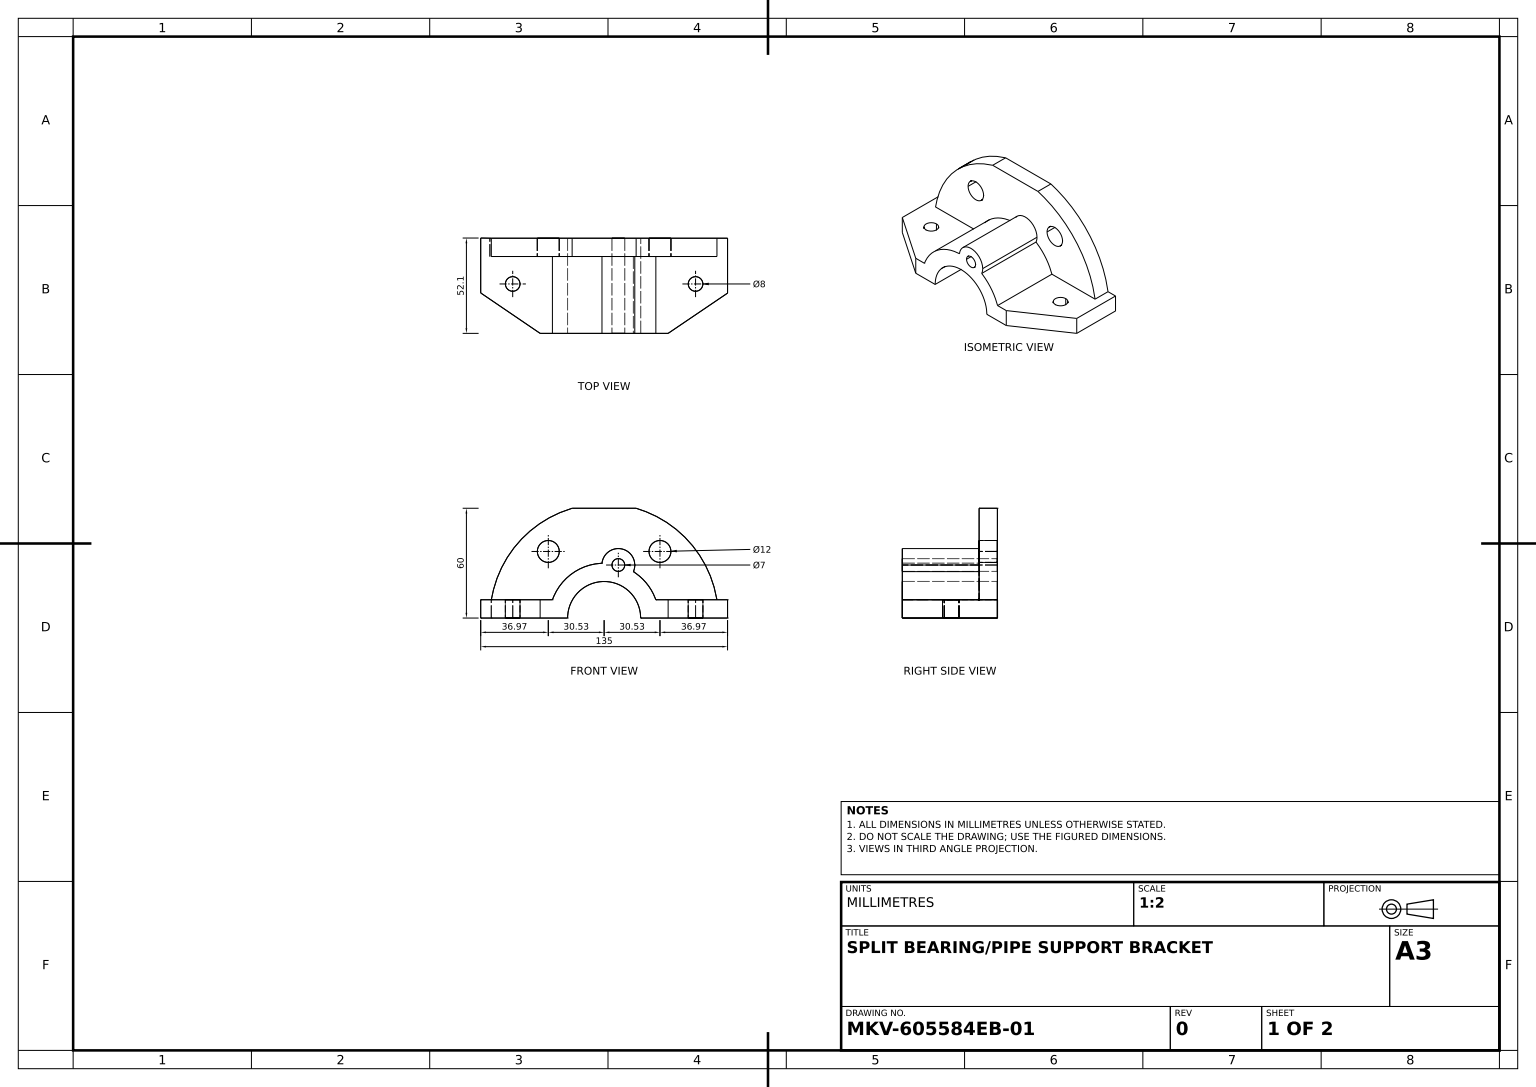
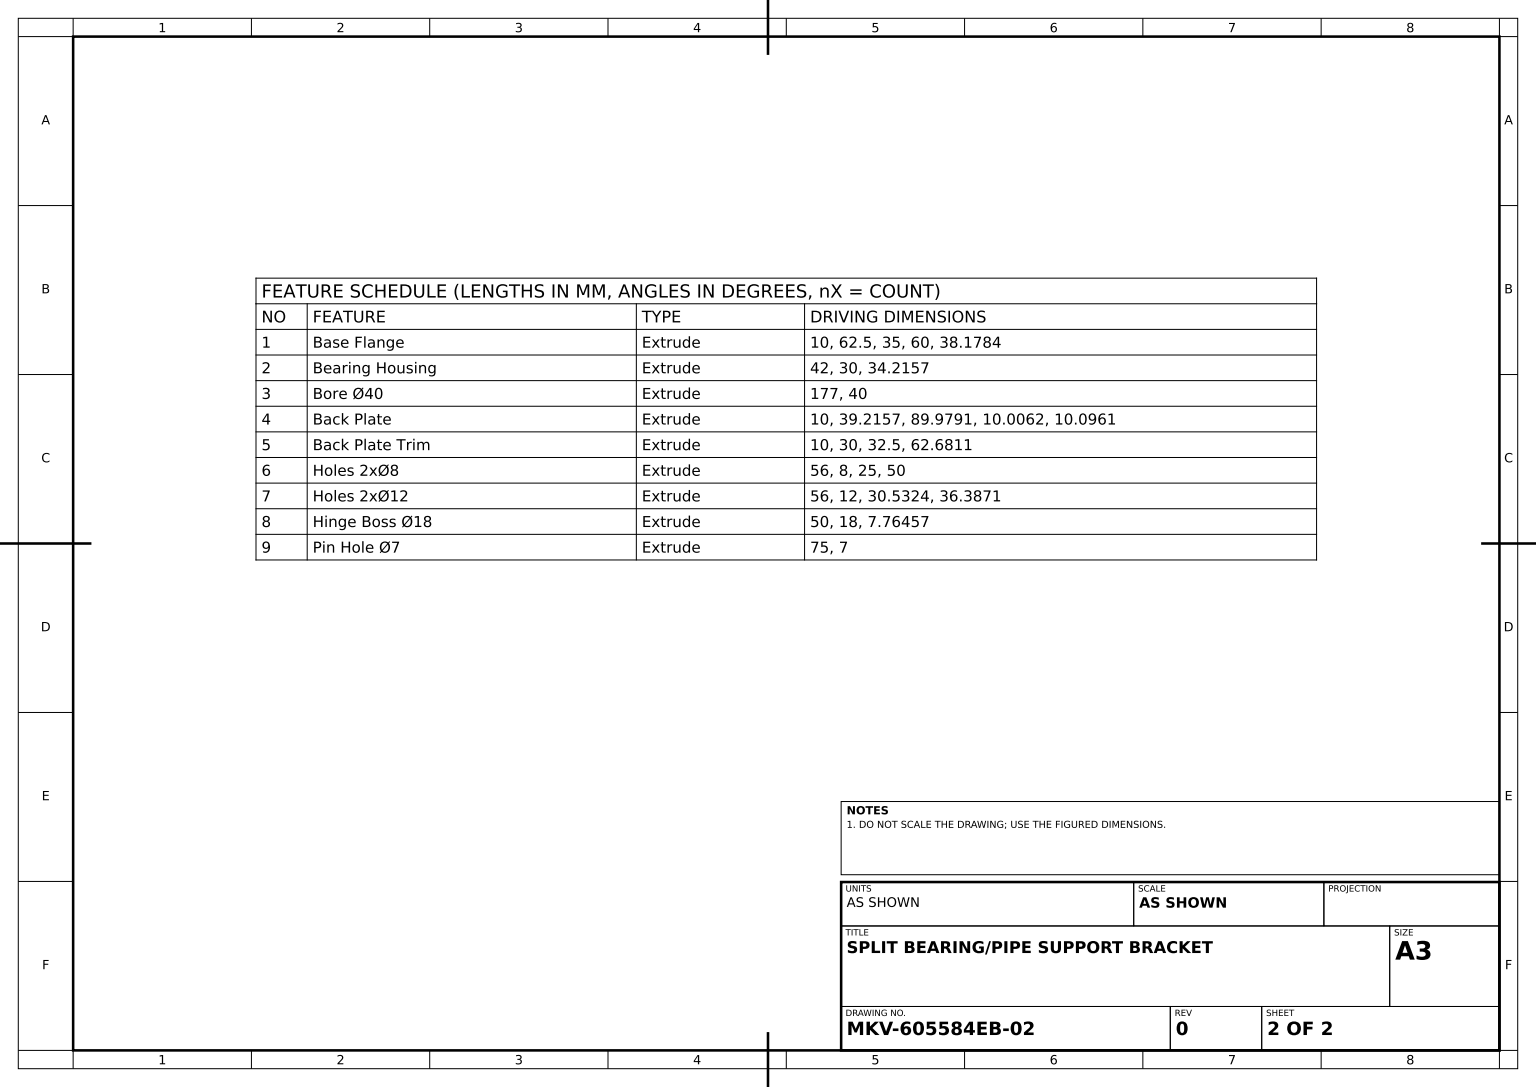
from build123d import *

# Parameters (mm, degrees)
BASE_FLANGE_DEPTH      = 10
BEARING_HOUSING_DEPTH  = 42
BORE_40_SKETCH_R       = 20
BORE_40_DEPTH          = 177
BACK_PLATE_DEPTH       = 10
BACK_PLATE_TRIM_DEPTH  = 10
HOLES_2X_8_SKETCH_R    = 4
HOLES_2X_8_DEPTH       = 56
HOLES_2X_12_SKETCH_R   = 6
HOLES_2X_12_DEPTH      = 56
HINGE_BOSS_18_SKETCH_R = 9
HINGE_BOSS_18_DEPTH    = 50
PIN_HOLE_7_SKETCH_R    = 3.5
PIN_HOLE_7_DEPTH       = 75


with BuildPart() as part:
    # Base Flange Sketch → Base Flange (new body)
    with BuildSketch(Plane.XY):
        with BuildLine():
            Line((-62.5, 0), (0, 0))
            Line((0, 0), (38.178366278, 0))
            Line((38.178366278, 0), (62.5, 0))
            ThreePointArc((62.5, 0), (50, 37.5), (17.5, 60))
            Line((17.5, 60), (0, 60))
            Line((0, 60), (-17.5, 60))
            ThreePointArc((-17.5, 60), (-50, 37.5), (-62.5, 0))
        make_face()
    extrude(amount=BASE_FLANGE_DEPTH)

    # Bearing Housing Sketch → Bearing Housing (add)
    with BuildSketch(Plane.XY.offset(10)):
        with BuildLine():
            Line((30, 0), (62.5, 0))
            ThreePointArc((62.5, 0), (62.298378138, 5.016181951), (61.694813396, 10))
            Line((61.694813396, 10), (28.284271247, 10))
            ThreePointArc((28.284271247, 10), (29.56795679, 5.073059362), (30, 0))
        make_face()
        with BuildLine():
            Line((-30, 0), (30, 0))
            ThreePointArc((30, 0), (29.56795679, 5.073059362), (28.284271247, 10))
            ThreePointArc((28.284271247, 10), (0, 30), (-28.284271247, 10))
            ThreePointArc((-28.284271247, 10), (-29.56795679, 5.073059362), (-30, 0))
        make_face()
        with BuildLine():
            Line((-62.5, 0), (-30, 0))
            ThreePointArc((-30, 0), (-29.56795679, 5.073059362), (-28.284271247, 10))
            Line((-28.284271247, 10), (-61.694813396, 10))
            ThreePointArc((-61.694813396, 10), (-62.298378138, 5.016181951), (-62.5, 0))
        make_face()
    extrude(amount=BEARING_HOUSING_DEPTH)

    # Bore Ø40 Sketch → Bore Ø40 (cut)
    with BuildSketch(Plane.XY.offset(52)):
        Circle(BORE_40_SKETCH_R)
    extrude(amount=-BORE_40_DEPTH, mode=Mode.SUBTRACT)

    # Back Plate Sketch → Back Plate (add)
    with BuildSketch(Plane(origin=(0, 10, 0), x_dir=(1, 0, 0), z_dir=(0, 1, 0))):
        Polygon((61.694813396, -52), (67.5, -52), (67.5, 0), (62.5, 0), (61.694813396, 0), align=None)
        Polygon((-67.5, -52), (-61.694813396, -52), (-61.694813396, 0.006233525), (-67.5, 0.096123111), align=None)
    extrude(amount=-BACK_PLATE_DEPTH)

    # Back Plate Trim Sketch → Back Plate Trim (cut)
    with BuildSketch(Plane(origin=(0, 10, 0), x_dir=(1, 0, 0), z_dir=(0, 1, 0))):
        Polygon((67.5, -30), (35, -52), (67.5, -52), align=None)
        Polygon((-67.5, -52), (-67.5, -29.903876889), (-35, -52), align=None)
    extrude(amount=-BACK_PLATE_TRIM_DEPTH, mode=Mode.SUBTRACT)

    # Holes 2xØ8 Sketch → Holes 2xØ8 (cut)
    with BuildSketch(Plane(origin=(0, 10, 0), x_dir=(1, 0, 0), z_dir=(0, 1, 0))):
        with Locations(Location((50, -25, 0), (0, 0, 270))):
            Circle(HOLES_2X_8_SKETCH_R)
        with Locations(Location((-50, -25, 0), (0, 0, 180))):
            Circle(HOLES_2X_8_SKETCH_R)
    extrude(amount=-HOLES_2X_8_DEPTH, mode=Mode.SUBTRACT)

    # Holes 2xØ12 Sketch → Holes 2xØ12 (cut)
    with BuildSketch(Plane.XY.offset(10)):
        with Locations((30.53241146, 36.387111048)):
            Circle(HOLES_2X_12_SKETCH_R)
        with Locations((-30.53241146, 36.387111048)):
            Circle(HOLES_2X_12_SKETCH_R)
    extrude(amount=-HOLES_2X_12_DEPTH, mode=Mode.SUBTRACT)

    # Hinge Boss Ø18 Sketch → Hinge Boss Ø18 (add)
    with BuildSketch(Plane.XY.offset(52)):
        with Locations((7.764571353, 28.977774789)):
            Circle(HINGE_BOSS_18_SKETCH_R)
    extrude(amount=-HINGE_BOSS_18_DEPTH)

    # Pin Hole Ø7 Sketch → Pin Hole Ø7 (cut)
    with BuildSketch(Plane.XY.offset(52)):
        with Locations((7.764571353, 28.977774789)):
            Circle(PIN_HOLE_7_SKETCH_R)
    extrude(amount=-PIN_HOLE_7_DEPTH, mode=Mode.SUBTRACT)


solid = part.part
